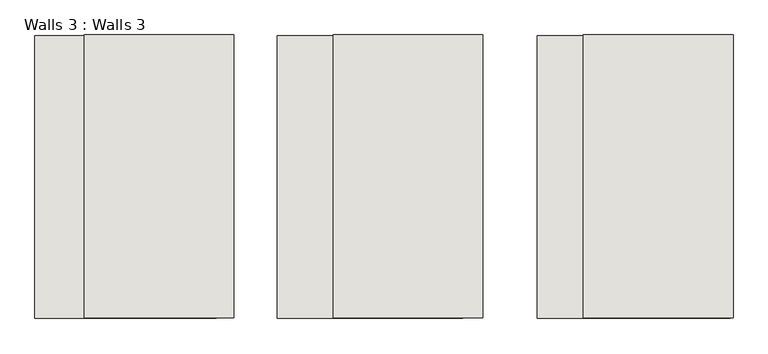
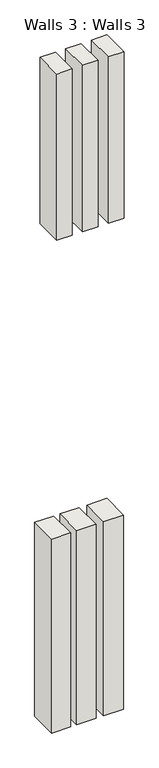
"""IFC4 building model written with IfcOpenShell, lengths in millimetres: wall geometry, Walls 3 : Walls 3."""

from ifc_helpers import new_model, si_unit, frame, origin, place, context, project, spatial, polyline, outline, extrude, source, transform, mapped, element, save


def walls_3_walls_3_caf9bd33(model_context):
    return source(origin(), model_context, "Body", "SweptSolid", [
        extrude(outline(polyline([(-5418.4712231, 815.4548476), (-5695.7432037, 815.4548476), (-5695.7432037, 1247.2548743), (-5418.4712231, 1247.2548743), (-5418.4712231, 815.4548476)])), frame((0.0, 0.0, 3962.4), z_axis=(0.0, 0.0, 1.0), x_axis=(1.0, 0.0, 0.0)), (0.0, 0.0, 1.0), 3019.7464127),
        extrude(outline(polyline([(-5041.8699124, 815.4548476), (-5325.3003942, 815.4548476), (-5325.3003942, 1247.2548743), (-5041.8699124, 1247.2548743), (-5041.8699124, 815.4548476)])), frame((0.0, 0.0, 3962.4), z_axis=(0.0, 0.0, 1.0), x_axis=(1.0, 0.0, 0.0)), (0.0, 0.0, 1.0), 3019.7464127),
        extrude(outline(polyline([(-4633.5386277, 815.4548476), (-4928.4445555, 815.4548476), (-4928.4445555, 1247.2548743), (-4633.5386277, 1247.2548743), (-4633.5386277, 815.4548476)])), frame((0.0, 0.0, 3962.4), z_axis=(0.0, 0.0, 1.0), x_axis=(1.0, 0.0, 0.0)), (0.0, 0.0, 1.0), 3019.7464127),
        extrude(outline(polyline([(-5392.0840532, 815.4548476), (-5620.6840532, 815.4548476), (-5620.6840532, 1247.2548743), (-5392.0840532, 1247.2548743), (-5392.0840532, 815.4548476)])), frame((0.0, 0.0, 11606.5141302), z_axis=(0.0, 0.0, 1.0), x_axis=(1.0, 0.0, 0.0)), (0.0, 0.0, 1.0), 2590.8),
        extrude(outline(polyline([(-4628.9432037, 815.4548476), (-4857.5432037, 815.4548476), (-4857.5432037, 1247.2548743), (-4628.9432037, 1247.2548743), (-4628.9432037, 815.4548476)])), frame((0.0, 0.0, 11606.5141302), z_axis=(0.0, 0.0, 1.0), x_axis=(1.0, 0.0, 0.0)), (0.0, 0.0, 1.0), 2590.8),
        extrude(outline(polyline([(-5011.0840532, 815.4548476), (-5239.6840532, 815.4548476), (-5239.6840532, 1247.2548743), (-5011.0840532, 1247.2548743), (-5011.0840532, 815.4548476)])), frame((0.0, 0.0, 11606.5141302), z_axis=(0.0, 0.0, 1.0), x_axis=(1.0, 0.0, 0.0)), (0.0, 0.0, 1.0), 2590.8),
    ])


if __name__ == "__main__":
    model = new_model("IFC4")
    model_context = context("Model", 3, world=origin())
    ifc_project = project(units=[si_unit("LENGTHUNIT", "METRE", prefix="MILLI")], contexts=[model_context])
    site = spatial("IfcSite", under=ifc_project)
    building = spatial("IfcBuilding", under=site)
    placement = place(None, origin())
    walls_3_walls_3_shape = walls_3_walls_3_caf9bd33(model_context)
    element("IfcWall", 1, ObjectType="Walls 3 : Walls 3", at=placement, inside=building, context=model_context, shape_type="MappedRepresentation", body=[
        mapped(walls_3_walls_3_shape, transform((0.0, 0.0, 0.0), x_axis=(1.0, 0.0, 0.0), y_axis=(0.0, 1.0, 0.0), z_axis=(0.0, 0.0, 1.0))),
    ])
    save(model, "model.ifc")

# Revit data of these elements
# Element 1 (IfcWall, "Walls 3 : Walls 3")
#   Materials on its faces: "Default Wall"
# Materials
#   "Default Wall": colour RGB 128 128 128, transparency 0
